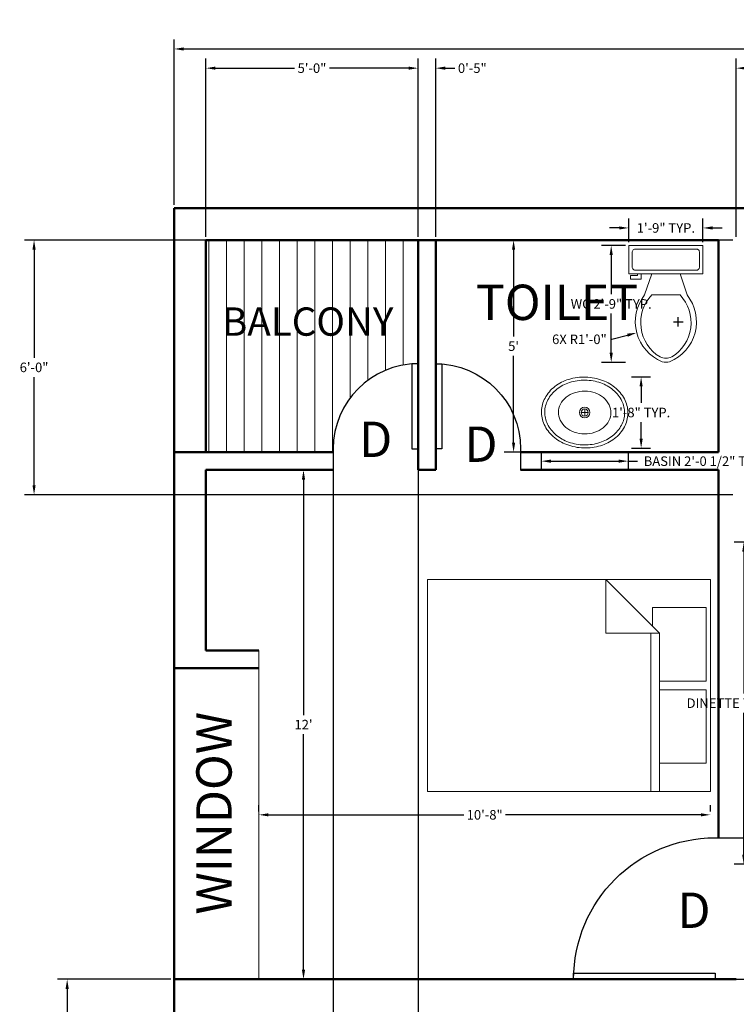
# Model space of a CAD drawing. Units: inches. Extents: x -15 to 796, y 111 to 651.
# Tile 3 of 6: x -13 to 189, y 373 to 651. Entities that reach past the tile are written whole.
import ezdxf

# ---------------------------------------------------------------- set-up
doc = ezdxf.new("R2010")
doc.units = ezdxf.units.IN
doc.header["$MEASUREMENT"] = 0
doc.layers.get('0').update_dxf_attribs({"color": 1})
for name, color, linetype, lineweight in [('A-ANNO-DIMS', 2, 'Continuous', 18), ('A-ANNO-TEXT', 7, 'Continuous', 18), ('A-AREA-IDEN', 7, 'Continuous', 25), ('A-DOOR', 3, 'Continuous', 25), ('A-FLOR-FIXT', 9, 'Continuous', 20), ('A-FLOR-PATT', 18, 'Continuous', 13), ('A-FURN', 8, 'Continuous', 18), ('A-GLAZ', 4, 'Continuous', 18), ('A-WALL', 7, 'Continuous', 50)]:
    doc.layers.add(name, color=color, linetype=linetype, lineweight=lineweight)
doc.styles.get("Standard").update_dxf_attribs({"font": 'arial.ttf'})
doc.dimstyles.get("Standard").update_dxf_attribs({"dimscale": 15, "dimtxt": 0.18, "dimasz": 0.18, "dimexe": 0.18, "dimexo": 0.0625, "dimgap": 0.09, "dimtad": 0, "dimtih": 1, "dimtoh": 1, "dimdec": 0, "dimzin": 0, "dimdsep": 46, "dimlunit": 3, "dimtxsty": 'Standard', "dimcen": 0.09, "dimadec": 0, "dimazin": 0, "dimtfac": 1, "dimtdec": 0, "dimtofl": 0, "dimtmove": 0, "dimatfit": 3, "dimfxl": 1, "dimtolj": 1, "dimtzin": 0, "dimarcsym": 0})

# ---------------------------------------------------------------- blocks, each defined once
blk = doc.blocks.new('Bed - Queen')
for p, q in [((0, -80.00003), (0, 0)), ((0, 0), (59.99999, 0)), ((59.99999, 0), (59.99999, -80.00003)), ((7.99999, -1.2), (28.79998, -1.2)), ((7.99999, -14.4), (7.99999, -1.2)), ((28.79998, -1.2), (28.79998, -14.4)), ((31.19999, -1.2), (51.99999, -1.2)), ((31.19999, -14.4), (31.19999, -1.2)), ((51.99999, -1.2), (51.99999, -16.4)), ((0, -14.4), (44.8, -14.4)), ((59.99999, -29.6), (44.8, -14.4)), ((44.8, -14.4), (44.8, -29.6)), ((51.99999, -16.4), (46.79936, -16.4)), ((44.8, -16.8), (0, -16.8)), ((44.8, -29.6), (59.99999, -29.6)), ((59.99999, -80.00003), (0, -80.00003))]:
    blk.add_line(p, q)
blk = doc.blocks.new('*U4')
for p, q in [((0, 0), (0, -6)), ((-40, 0), (-40, -6))]:
    blk.add_line(p, q)
blk.add_lwpolyline([(0, 0), (0, 40), (-1.75, 40), (-1.75, 0)], close=True)
blk.add_arc((0, 0), 40, 90, 180)
blk = doc.blocks.new('*U8')
for p, q in [((-24, 0), (-24, -6)), ((0, 0), (0, -6))]:
    blk.add_line(p, q)
blk.add_lwpolyline([(0, 0), (0, 24), (-1.75, 24), (-1.75, 0)], close=True)
blk.add_arc((0, 0), 24, 90, 180)
blk = doc.blocks.new('Sink - Oval top')
for p, q in [((-1, 0), (1, 0)), ((0, 1), (0, -1))]:
    blk.add_line(p, q)
for points in [[(-12.23, 0.39, 0.117634), (-11.46, -3.36, 0.104469), (-8.88, -6.8, 0.090016), (-5.08, -9.07, 0.08192), (-0.32, -10.02, 0.08192), (4.49, -9.38, 0.090016), (8.42, -7.36, 0.104469), (11.22, -4.09, 0.117634), (12.23, -0.39, 0.117634), (11.46, 3.36, 0.104469), (8.88, 6.8, 0.090016), (5.08, 9.07, 0.08192), (0.32, 10.02, 0.08192), (-4.49, 9.38, 0.090016), (-8.42, 7.36, 0.104469), (-11.22, 4.09, 0.117634)], [(-11.29, 0.16, 0.118622), (-10.52, -3.25, 0.104678), (-8.07, -6.36, 0.089562), (-4.54, -8.37, 0.081185), (-0.13, -9.15, 0.081185), (4.3, -8.49, 0.089562), (7.89, -6.58, 0.104678), (10.42, -3.55, 0.118622), (11.29, -0.16, 0.118622), (10.52, 3.25, 0.104678), (8.07, 6.36, 0.089562), (4.54, 8.37, 0.081185), (0.13, 9.15, 0.081185), (-4.3, 8.49, 0.089562), (-7.89, 6.58, 0.104678), (-10.42, 3.55, 0.118622)], [(-7.42, 0.08, 0.118283), (-6.91, -2.17, 0.104607), (-5.29, -4.21, 0.089718), (-2.97, -5.53, 0.081436), (-0.07, -6.04, 0.081436), (2.84, -5.59, 0.089718), (5.2, -4.33, 0.104607), (6.86, -2.32, 0.118283), (7.42, -0.08, 0.118283), (6.91, 2.17, 0.104607), (5.29, 4.21, 0.089718), (2.97, 5.53, 0.081436), (0.07, 6.04, 0.081436), (-2.84, 5.59, 0.089718), (-5.2, 4.33, 0.104607), (-6.86, 2.32, 0.118283)]]:
    blk.add_lwpolyline(points, format="xyb", close=True)
for radius in [1.5, 1]:
    blk.add_circle((0, 0), radius)
blk = doc.blocks.new('Toilet - top')
for p, q in [((9.5, -6), (9.5, -2)), ((-8, -8.5), (-8, -8)), ((-7, -8), (-7, -9.5)), ((-4, -8), (-6, -14)), ((4, -8), (6, -14)), ((-10, -8.5), (-8, -8.5)), ((-10, -9.5), (-10, -8.5)), ((-7, -9.5), (-10, -9.5)), ((4, -14), (-4, -14))]:
    blk.add_line(p, q)
blk.add_lwpolyline([(10.5, -8), (10.5, 0), (-10.5, 0), (-10.5, -8)], close=True)
for points in [[(-9.5, -2), (-9.5, -6)], [(8.5, -1), (-8.5, -1)], [(-8.5, -7), (8.5, -7)]]:
    blk.add_lwpolyline(points)
for centre, radius, start, end in [((-8.62, -1.88), 0.884, 81.8699, 188.1301), ((8.62, -1.88), 0.884, 351.8699, 98.1301), ((-8.62, -6.12), 0.884, 171.8699, 278.1301), ((8.62, -6.12), 0.884, 261.8699, 8.1301), ((3.52, -21.58), 12.17, 141.4691, 247.9714), ((4.2, -21.82), 11.33, 136.3677, 238.9468), ((-3.52, -21.58), 12.17, 292.0284, 38.5307), ((-4.2, -21.82), 11.33, 301.053, 43.6321), ((0, -27.88), 4, 245.7318, 294.2682), ((0, -29), 4, 254.8605, 285.1395)]:
    blk.add_arc(centre, radius, start, end)
blk = doc.blocks.new('*D16')
at = {"layer": 'A-ANNO-DIMS', "color": 0, "lineweight": -2, "transparency": 16777216}
for p, q in [((30.18, 599.06), (30.18, 645.85)), ((697.18, 599.06), (697.18, 645.85)), ((32.88, 643.15), (336.57, 643.15)), ((694.48, 643.15), (390.8, 643.15))]:
    blk.add_line(p, q, dxfattribs=at)
at = {"layer": 'A-ANNO-DIMS', "color": 0, "transparency": 16777216}
for points in [[(32.88, 643.6), (32.88, 642.7), (30.18, 643.15)], [(694.48, 643.6), (694.48, 642.7), (697.18, 643.15)]]:
    blk.add_solid(points, dxfattribs=at)
at = {"layer": 'Defpoints', "color": 0, "transparency": 16777216}
for p in [(697.18, 643.15), (30.18, 598.13), (697.18, 598.13)]:
    blk.add_point(p, dxfattribs=at)
at = {"layer": 'A-ANNO-DIMS', "color": 0, "transparency": 16777216, "insert": (363.68, 643.15), "char_height": 2.7, "attachment_point": 5}
blk.add_mtext('\\A1;{\\H5.55556x;55\'-7"}', dxfattribs=at)
blk = doc.blocks.new('*D19')
at = {"layer": 'A-ANNO-DIMS', "color": 0, "lineweight": -2, "transparency": 16777216}
for p, q in [((29.24, 380.13), (-2.76, 380.13)), ((-0.06, 377.43), (-0.06, 306.36)), ((-0.06, 229.83), (-0.06, 300.9)), ((29.24, 227.13), (-2.76, 227.13))]:
    blk.add_line(p, q, dxfattribs=at)
at = {"layer": 'A-ANNO-DIMS', "color": 0, "transparency": 16777216}
for points in [[(-0.51, 377.43), (0.39, 377.43), (-0.06, 380.13)], [(-0.51, 229.83), (0.39, 229.83), (-0.06, 227.13)]]:
    blk.add_solid(points, dxfattribs=at)
at = {"layer": 'Defpoints', "color": 0, "transparency": 16777216}
for p in [(30.18, 380.13), (-0.06, 227.13), (30.18, 227.13)]:
    blk.add_point(p, dxfattribs=at)
at = {"layer": 'A-ANNO-DIMS', "color": 0, "transparency": 16777216, "insert": (-0.06, 303.63), "char_height": 2.7, "attachment_point": 5}
blk.add_mtext('\\A1;12\'-9"', dxfattribs=at)
blk = doc.blocks.new('*D23')
at = {"layer": 'A-ANNO-DIMS', "color": 0, "lineweight": -2, "transparency": 16777216}
for p, q in [((141.7, 589.13), (123.49, 589.13)), ((126.19, 586.43), (126.19, 561.85)), ((126.19, 531.83), (126.19, 556.4)), ((141.7, 529.13), (123.49, 529.13))]:
    blk.add_line(p, q, dxfattribs=at)
at = {"layer": 'A-ANNO-DIMS', "color": 0, "transparency": 16777216}
for points in [[(125.74, 586.43), (126.64, 586.43), (126.19, 589.13)], [(125.74, 531.83), (126.64, 531.83), (126.19, 529.13)]]:
    blk.add_solid(points, dxfattribs=at)
at = {"layer": 'Defpoints', "color": 0, "transparency": 16777216}
for p in [(142.63, 589.13), (126.19, 529.13), (142.63, 529.13)]:
    blk.add_point(p, dxfattribs=at)
at = {"layer": 'A-ANNO-DIMS', "color": 0, "transparency": 16777216, "insert": (126.19, 559.13), "char_height": 2.7, "attachment_point": 5}
blk.add_mtext("\\A1;5'", dxfattribs=at)
blk = doc.blocks.new('*D24')
at = {"layer": 'A-ANNO-DIMS', "color": 0, "lineweight": -2, "transparency": 16777216}
for p, q in [((74.24, 524.13), (64.08, 524.13)), ((66.78, 521.43), (66.78, 454.83)), ((66.78, 382.83), (66.78, 449.42)), ((74.24, 380.13), (64.08, 380.13))]:
    blk.add_line(p, q, dxfattribs=at)
at = {"layer": 'A-ANNO-DIMS', "color": 0, "transparency": 16777216}
for points in [[(66.33, 521.43), (67.23, 521.43), (66.78, 524.13)], [(66.33, 382.83), (67.23, 382.83), (66.78, 380.13)]]:
    blk.add_solid(points, dxfattribs=at)
at = {"layer": 'Defpoints', "color": 0, "transparency": 16777216}
for p in [(75.18, 524.13), (66.78, 380.13), (75.18, 380.13)]:
    blk.add_point(p, dxfattribs=at)
at = {"layer": 'A-ANNO-DIMS', "color": 0, "transparency": 16777216, "insert": (66.78, 452.13), "char_height": 2.7, "attachment_point": 5}
blk.add_mtext("\\A1;12'", dxfattribs=at)
blk = doc.blocks.new('*D25')
at = {"layer": 'A-ANNO-DIMS', "color": 0, "lineweight": -2, "transparency": 16777216}
for p, q in [((54.18, 427.56), (54.18, 429.33)), ((181.85, 427.56), (181.85, 429.33)), ((56.88, 426.63), (112.16, 426.63)), ((179.15, 426.63), (123.88, 426.63))]:
    blk.add_line(p, q, dxfattribs=at)
at = {"layer": 'A-ANNO-DIMS', "color": 0, "transparency": 16777216}
for points in [[(56.88, 427.08), (56.88, 426.18), (54.18, 426.63)], [(179.15, 427.08), (179.15, 426.18), (181.85, 426.63)]]:
    blk.add_solid(points, dxfattribs=at)
at = {"layer": 'Defpoints', "color": 0, "transparency": 16777216}
for p in [(54.18, 426.63), (181.85, 426.63), (181.85, 426.63)]:
    blk.add_point(p, dxfattribs=at)
at = {"layer": 'A-ANNO-DIMS', "color": 0, "transparency": 16777216, "insert": (118.02, 426.63), "char_height": 2.7, "attachment_point": 5}
blk.add_mtext('\\A1;10\'-8"', dxfattribs=at)
blk = doc.blocks.new('*D45')
at = {"layer": 'A-ANNO-DIMS', "color": 0, "lineweight": -2, "transparency": 16777216}
for p, q in [((134.03, 529.37), (134.03, 523.92)), ((158.58, 529.37), (158.58, 523.92)), ((136.73, 526.62), (155.88, 526.62)), ((158.58, 526.62), (161.28, 526.62))]:
    blk.add_line(p, q, dxfattribs=at)
at = {"layer": 'A-ANNO-DIMS', "color": 0, "transparency": 16777216}
for points in [[(136.73, 527.07), (136.73, 526.17), (134.03, 526.62)], [(155.88, 527.07), (155.88, 526.17), (158.58, 526.62)]]:
    blk.add_solid(points, dxfattribs=at)
at = {"layer": 'Defpoints', "color": 0, "transparency": 16777216}
for p in [(134.03, 530.3), (158.58, 530.3), (158.58, 526.62)]:
    blk.add_point(p, dxfattribs=at)
at = {"layer": 'A-ANNO-DIMS', "color": 0, "transparency": 16777216, "insert": (180.13, 526.62), "char_height": 2.7, "attachment_point": 5}
blk.add_mtext('\\A1;BASIN 2\'-0 1/2" TYP.', dxfattribs=at)
blk = doc.blocks.new('*D46')
at = {"layer": 'A-ANNO-DIMS', "color": 0, "lineweight": -2, "transparency": 16777216}
for p, q in [((159.51, 550.44), (164.96, 550.44)), ((162.26, 547.74), (162.26, 543.1)), ((162.26, 533), (162.26, 537.64)), ((159.51, 530.3), (164.96, 530.3))]:
    blk.add_line(p, q, dxfattribs=at)
at = {"layer": 'A-ANNO-DIMS', "color": 0, "transparency": 16777216}
for points in [[(161.81, 547.74), (162.71, 547.74), (162.26, 550.44)], [(161.81, 533), (162.71, 533), (162.26, 530.3)]]:
    blk.add_solid(points, dxfattribs=at)
at = {"layer": 'Defpoints', "color": 0, "transparency": 16777216}
for p in [(158.58, 550.44), (162.26, 550.44), (158.58, 530.3)]:
    blk.add_point(p, dxfattribs=at)
at = {"layer": 'A-ANNO-DIMS', "color": 0, "transparency": 16777216, "insert": (162.26, 540.37), "char_height": 2.7, "attachment_point": 5}
blk.add_mtext('\\A1;1\'-8" TYP.', dxfattribs=at)
blk = doc.blocks.new('*D47')
at = {"layer": 'A-ANNO-DIMS', "color": 0, "lineweight": -2, "transparency": 16777216}
for p, q in [((157.82, 587.6), (151.1, 587.6)), ((153.8, 584.9), (153.8, 573.82)), ((153.8, 557.25), (153.8, 568.33)), ((157.82, 554.55), (151.1, 554.55))]:
    blk.add_line(p, q, dxfattribs=at)
at = {"layer": 'A-ANNO-DIMS', "color": 0, "transparency": 16777216}
for points in [[(153.35, 584.9), (154.25, 584.9), (153.8, 587.6)], [(153.35, 557.25), (154.25, 557.25), (153.8, 554.55)]]:
    blk.add_solid(points, dxfattribs=at)
at = {"layer": 'Defpoints', "color": 0, "transparency": 16777216}
for p in [(153.8, 587.6), (158.76, 587.6), (158.76, 554.55)]:
    blk.add_point(p, dxfattribs=at)
at = {"layer": 'A-ANNO-DIMS', "color": 0, "transparency": 16777216, "insert": (153.8, 571.07), "char_height": 2.7, "attachment_point": 5}
blk.add_mtext('\\A1;WC 2\'-9" TYP.', dxfattribs=at)
blk = doc.blocks.new('*D48')
at = {"layer": 'A-ANNO-DIMS', "color": 0, "lineweight": -2, "transparency": 16777216}
for p, q in [((158.76, 588.54), (158.76, 595.25)), ((179.76, 588.54), (179.76, 595.25)), ((156.06, 592.55), (153.36, 592.55)), ((182.46, 592.55), (185.16, 592.55))]:
    blk.add_line(p, q, dxfattribs=at)
at = {"layer": 'A-ANNO-DIMS', "color": 0, "transparency": 16777216}
for points in [[(156.06, 593), (156.06, 592.1), (158.76, 592.55)], [(182.46, 593), (182.46, 592.1), (179.76, 592.55)]]:
    blk.add_solid(points, dxfattribs=at)
at = {"layer": 'Defpoints', "color": 0, "transparency": 16777216}
for p in [(179.76, 592.55), (158.76, 587.6), (179.76, 587.6)]:
    blk.add_point(p, dxfattribs=at)
at = {"layer": 'A-ANNO-DIMS', "color": 0, "transparency": 16777216, "insert": (169.26, 592.55), "char_height": 2.7, "attachment_point": 5}
blk.add_mtext('\\A1;1\'-9" TYP.', dxfattribs=at)
blk = doc.blocks.new('*D55')
at = {"layer": 'A-ANNO-DIMS', "color": 0, "lineweight": -2, "transparency": 16777216}
for p, q in [((204, 503.69), (188.59, 503.69)), ((191.29, 500.99), (191.29, 460.89)), ((191.29, 415.39), (191.29, 455.48)), ((204, 412.69), (188.59, 412.69))]:
    blk.add_line(p, q, dxfattribs=at)
at = {"layer": 'A-ANNO-DIMS', "color": 0, "transparency": 16777216}
for points in [[(190.84, 500.99), (191.74, 500.99), (191.29, 503.69)], [(190.84, 415.39), (191.74, 415.39), (191.29, 412.69)]]:
    blk.add_solid(points, dxfattribs=at)
at = {"layer": 'Defpoints', "color": 0, "transparency": 16777216}
for p in [(204.94, 503.69), (191.29, 412.69), (204.94, 412.69)]:
    blk.add_point(p, dxfattribs=at)
at = {"layer": 'A-ANNO-DIMS', "color": 0, "transparency": 16777216, "insert": (191.29, 458.19), "char_height": 2.7, "attachment_point": 5}
blk.add_mtext('\\A1;DINETTE 7\'-7" TYP.', dxfattribs=at)
blk = doc.blocks.new('*D70')
at = {"layer": 'A-ANNO-DIMS', "color": 0, "lineweight": -2, "transparency": 16777216}
for p, q in [((39.18, 590.06), (39.18, 640.43)), ((99.18, 590.06), (99.18, 640.43)), ((41.88, 637.73), (64.24, 637.73)), ((96.48, 637.73), (74.12, 637.73))]:
    blk.add_line(p, q, dxfattribs=at)
at = {"layer": 'A-ANNO-DIMS', "color": 0, "transparency": 16777216}
for points in [[(41.88, 638.18), (41.88, 637.28), (39.18, 637.73)], [(96.48, 638.18), (96.48, 637.28), (99.18, 637.73)]]:
    blk.add_solid(points, dxfattribs=at)
at = {"layer": 'Defpoints', "color": 0, "transparency": 16777216}
for p in [(99.18, 637.73), (39.18, 589.13), (99.18, 589.13)]:
    blk.add_point(p, dxfattribs=at)
at = {"layer": 'A-ANNO-DIMS', "color": 0, "transparency": 16777216, "insert": (69.18, 637.73), "char_height": 2.7, "attachment_point": 5}
blk.add_mtext('\\A1;5\'-0"', dxfattribs=at)
blk = doc.blocks.new('*D71')
at = {"layer": 'A-ANNO-DIMS', "color": 0, "lineweight": -2, "transparency": 16777216}
for p, q in [((188.24, 589.13), (-12.12, 589.13)), ((-9.42, 586.43), (-9.42, 555.86)), ((-9.42, 519.83), (-9.42, 550.4)), ((188.24, 517.13), (-12.12, 517.13))]:
    blk.add_line(p, q, dxfattribs=at)
at = {"layer": 'A-ANNO-DIMS', "color": 0, "transparency": 16777216}
for points in [[(-9.87, 586.43), (-8.97, 586.43), (-9.42, 589.13)], [(-9.87, 519.83), (-8.97, 519.83), (-9.42, 517.13)]]:
    blk.add_solid(points, dxfattribs=at)
at = {"layer": 'Defpoints', "color": 0, "transparency": 16777216}
for p in [(189.18, 589.13), (-9.42, 517.13), (189.18, 517.13)]:
    blk.add_point(p, dxfattribs=at)
at = {"layer": 'A-ANNO-DIMS', "color": 0, "transparency": 16777216, "insert": (-9.42, 553.13), "char_height": 2.7, "attachment_point": 5}
blk.add_mtext('\\A1;6\'-0"', dxfattribs=at)
blk = doc.blocks.new('*D76')
at = {"layer": 'A-ANNO-DIMS', "color": 0, "lineweight": -2, "transparency": 16777216}
for p, q in [((189.18, 590.06), (189.18, 640.43)), ((231.37, 599.06), (231.37, 640.43)), ((191.88, 637.73), (205.34, 637.73)), ((228.67, 637.73), (215.21, 637.73))]:
    blk.add_line(p, q, dxfattribs=at)
at = {"layer": 'A-ANNO-DIMS', "color": 0, "transparency": 16777216}
for points in [[(191.88, 638.18), (191.88, 637.28), (189.18, 637.73)], [(228.67, 638.18), (228.67, 637.28), (231.37, 637.73)]]:
    blk.add_solid(points, dxfattribs=at)
at = {"layer": 'Defpoints', "color": 0, "transparency": 16777216}
for p in [(231.37, 637.73), (231.37, 598.13), (189.18, 589.13)]:
    blk.add_point(p, dxfattribs=at)
at = {"layer": 'A-ANNO-DIMS', "color": 0, "transparency": 16777216, "insert": (210.27, 637.73), "char_height": 2.7, "attachment_point": 5}
blk.add_mtext('\\A1;3\'-6"', dxfattribs=at)
blk = doc.blocks.new('*D78')
at = {"layer": 'A-ANNO-DIMS', "color": 0, "lineweight": -2, "transparency": 16777216}
for p, q in [((185.12, 420.13), (739.48, 420.13)), ((736.78, 417.43), (736.78, 402.86)), ((736.78, 382.83), (736.78, 397.4)), ((185.87, 380.13), (739.48, 380.13))]:
    blk.add_line(p, q, dxfattribs=at)
at = {"layer": 'A-ANNO-DIMS', "color": 0, "transparency": 16777216}
for points in [[(736.33, 417.43), (737.23, 417.43), (736.78, 420.13)], [(736.33, 382.83), (737.23, 382.83), (736.78, 380.13)]]:
    blk.add_solid(points, dxfattribs=at)
at = {"layer": 'Defpoints', "color": 0, "transparency": 16777216}
for p in [(184.18, 420.13), (736.78, 420.13), (184.93, 380.13)]:
    blk.add_point(p, dxfattribs=at)
at = {"layer": 'A-ANNO-DIMS', "color": 0, "transparency": 16777216, "insert": (736.78, 400.13), "char_height": 2.7, "attachment_point": 5}
blk.add_mtext('\\A1;3\'-4"', dxfattribs=at)
blk = doc.blocks.new('*D80')
at = {"layer": 'A-ANNO-DIMS', "color": 0, "lineweight": -2, "transparency": 16777216}
for p, q in [((75.18, 528.19), (75.18, 125.83)), ((99.18, 527.44), (99.18, 125.83)), ((77.88, 128.53), (82.22, 128.53)), ((96.48, 128.53), (92.14, 128.53))]:
    blk.add_line(p, q, dxfattribs=at)
at = {"layer": 'A-ANNO-DIMS', "color": 0, "transparency": 16777216}
for points in [[(77.88, 128.98), (77.88, 128.08), (75.18, 128.53)], [(96.48, 128.98), (96.48, 128.08), (99.18, 128.53)]]:
    blk.add_solid(points, dxfattribs=at)
at = {"layer": 'Defpoints', "color": 0, "transparency": 16777216}
for p in [(75.18, 529.13), (99.18, 528.38), (75.18, 128.53)]:
    blk.add_point(p, dxfattribs=at)
at = {"layer": 'A-ANNO-DIMS', "color": 0, "transparency": 16777216, "insert": (87.18, 128.53), "char_height": 2.7, "attachment_point": 5}
blk.add_mtext('\\A1;2\'-0"', dxfattribs=at)
blk = doc.blocks.new('*D82')
at = {"layer": 'A-ANNO-DIMS', "color": 0, "lineweight": -2, "transparency": 16777216}
for p, q in [((99.18, 590.06), (99.18, 640.43)), ((104.18, 590.06), (104.18, 640.43)), ((96.48, 637.73), (93.78, 637.73)), ((106.88, 637.73), (109.58, 637.73))]:
    blk.add_line(p, q, dxfattribs=at)
at = {"layer": 'A-ANNO-DIMS', "color": 0, "transparency": 16777216}
for points in [[(96.48, 638.18), (96.48, 637.28), (99.18, 637.73)], [(106.88, 638.18), (106.88, 637.28), (104.18, 637.73)]]:
    blk.add_solid(points, dxfattribs=at)
at = {"layer": 'Defpoints', "color": 0, "transparency": 16777216}
for p in [(104.18, 637.73), (99.18, 589.13), (104.18, 589.13)]:
    blk.add_point(p, dxfattribs=at)
at = {"layer": 'A-ANNO-DIMS', "color": 0, "transparency": 16777216, "insert": (114.52, 637.73), "char_height": 2.7, "attachment_point": 5}
blk.add_mtext('\\A1;0\'-5"', dxfattribs=at)
blk = doc.blocks.new('*D89')
at = {"layer": 'A-ANNO-DIMS', "color": 0, "lineweight": -2, "transparency": 16777216}
for p, q in [((171.43, 566.02), (174.13, 566.02)), ((172.78, 564.67), (172.78, 567.37)), ((153.95, 561.07), (158.4, 562.24))]:
    blk.add_line(p, q, dxfattribs=at)
at = {"layer": 'A-ANNO-DIMS', "color": 0, "transparency": 16777216}
blk.add_solid([(158.28, 562.67), (158.51, 561.8), (161.01, 562.92)], dxfattribs=at)
at = {"layer": 'Defpoints', "color": 0, "transparency": 16777216}
for p in [(172.78, 566.02), (161.01, 562.92)]:
    blk.add_point(p, dxfattribs=at)
at = {"layer": 'A-ANNO-DIMS', "color": 0, "transparency": 16777216, "insert": (144.81, 561.07), "char_height": 2.7, "attachment_point": 5}
blk.add_mtext('\\A1;6X R1\'-0"', dxfattribs=at)

msp = doc.modelspace()

# ---------------------------------------------------------------- hatches: boundary and pattern name
at = {"layer": 'A-FLOR-PATT'}
h = msp.add_hatch(dxfattribs=at)
h.set_pattern_fill('_USER', color=256, scale=5, angle=90, pattern_type=0)
h.set_pattern_definition([(90, (0, 0), (-5, 3e-16), [])])
h.paths.add_polyline_path([(99.18, 589.13), (39.18, 589.13), (39.18, 529.13), (75.18, 529.13), (75.18, 530.13, -0.392996), (97.43, 554.06), (97.43, 554.13), (99.18, 554.13)])
h.paths.add_polyline_path([(688.18, 589.13), (628.18, 589.13), (628.18, 554.13), (629.93, 554.13), (629.93, 554.06, -0.392996), (652.18, 530.13), (652.18, 529.13), (688.18, 529.13)])
h.paths.add_polyline_path([(40.9, 557.57), (98.32, 557.57), (98.32, 574.06), (40.9, 574.06)], flags=24)
h.paths.add_polyline_path([(628.32, 557.57), (685.73, 557.57), (685.73, 574.06), (628.32, 574.06)], flags=24)

# ---------------------------------------------------------------- linework, layer by layer
at = {"layer": 'A-GLAZ'}
msp.add_line((54.18, 473.13), (54.18, 380.13), dxfattribs=at)
at = {"layer": 'A-WALL'}
for p, q in [((30.18, 598.13), (30.18, 468.13)), ((322.48, 598.13), (30.18, 598.13)), ((39.18, 589.13), (39.18, 529.13)), ((184.18, 589.13), (39.18, 589.13)), ((99.18, 589.13), (99.18, 524.13)), ((104.18, 589.13), (104.18, 524.13)), ((184.18, 529.13), (184.18, 589.13)), ((39.18, 529.13), (30.18, 529.13)), ((75.18, 529.13), (39.18, 529.13)), ((184.18, 529.13), (128.18, 529.13)), ((39.18, 524.13), (39.18, 473.13)), ((75.18, 524.13), (39.18, 524.13)), ((104.18, 524.13), (99.18, 524.13)), ((184.18, 524.13), (128.18, 524.13)), ((184.18, 420.13), (184.18, 524.13)), ((54.18, 473.13), (39.18, 473.13)), ((30.18, 468.13), (30.18, 380.13)), ((54.18, 468.13), (30.18, 468.13)), ((30.18, 380.13), (30.18, 227.13)), ((189.18, 380.13), (30.18, 380.13))]:
    msp.add_line(p, q, dxfattribs=at)

# ---------------------------------------------------------------- block references
at = {"layer": 'A-DOOR'}
msp.add_blockref('*U8', (99.18, 530.13), dxfattribs=at)
at = {"layer": 'A-DOOR', "xscale": -1}
msp.add_blockref('*U8', (104.18, 530.13), dxfattribs=at)
at = {"layer": 'A-DOOR', "xscale": -1, "rotation": 90}
msp.add_blockref('*U4', (183.18, 380.13), dxfattribs=at)
at = {"layer": 'A-FLOR-FIXT'}
for name, p in [('Toilet - top', (169.26, 587.6)), ('Sink - Oval top', (146.3, 540.37))]:
    msp.add_blockref(name, p, dxfattribs=at)
at = {"layer": 'A-FURN', "xscale": -1, "rotation": 270}
msp.add_blockref('Bed - Queen', (181.85, 433.2), dxfattribs=at)

# ---------------------------------------------------------------- texts
at = {"layer": 'A-ANNO-TEXT'}
msp.add_text('WINDOW', height=10, rotation=90, dxfattribs=at).set_placement((46.46, 398.41))
at = {"layer": 'A-ANNO-TEXT', "char_height": 10, "attachment_point": 1}
for insert in [(82.5, 537.79), (112.27, 536.41), (172.51, 404.64)]:
    msp.add_mtext_dynamic_manual_height_columns('D', width=13.2435, gutter_width=1, heights=[0], dxfattribs=dict(at, insert=insert))
at = {"layer": 'A-AREA-IDEN', "attachment_point": 1}
for s, width, insert, char_height in [('TOILET', 20.6028, (115.54, 576.52), 10), ('BALCONY', 13.9372, (43.72, 570.08), 8)]:
    msp.add_mtext_dynamic_manual_height_columns(s, width=width, gutter_width=50, heights=[0], dxfattribs=dict(at, insert=insert, char_height=char_height))

# ---------------------------------------------------------------- dimensions: what is measured, and where the dimension line sits
at = {"layer": 'A-ANNO-DIMS'}
dim = msp.add_linear_dim(base=(697.18, 643.15), p1=(30.18, 598.13), p2=(697.18, 598.13), text='{\\H5.55556x;<>}', dimstyle='Standard', override={"dimclrd": 0, "dimclre": 0, "dimclrt": 0}, dxfattribs=at)
dim.commit()
dim.dimension.update_dxf_attribs({"geometry": '*D16', "text_midpoint": (363.68, 643.15), "dimtype": 160})
for base, p1, p2, override, picture, middle in [((99.18, 637.73), (39.18, 589.13), (99.18, 589.13), {"dimdec": 1, "dimlfac": 1, "dimrnd": 0, "dimzin": 1, "dimdsep": 46, "dimlunit": 4, "dimfrac": 2}, '*D70', (69.18, 637.73)), ((104.18, 637.73), (99.18, 589.13), (104.18, 589.13), {"dimdec": 1, "dimlfac": 1, "dimrnd": 0, "dimzin": 1, "dimdsep": 46, "dimlunit": 4, "dimfrac": 2}, '*D82', (114.52, 637.73)), ((231.37, 637.73), (189.18, 589.13), (231.37, 598.13), {"dimdec": 1, "dimlfac": 1, "dimrnd": 0, "dimzin": 1, "dimdsep": 46, "dimlunit": 4, "dimfrac": 2}, '*D76', (210.27, 637.73)), ((75.18, 128.53), (99.18, 528.38), (75.18, 529.13), {"dimdec": 1, "dimlfac": 1, "dimrnd": 0, "dimzin": 1, "dimdsep": 46, "dimlunit": 4, "dimfrac": 2}, '*D80', (87.18, 128.53)), ((181.85, 426.63), (54.18, 426.63), (181.85, 426.63), {"dimclrd": 0, "dimclre": 0, "dimclrt": 0}, '*D25', (118.02, 426.63))]:
    dim = msp.add_linear_dim(base=base, p1=p1, p2=p2, dimstyle='Standard', override=override, dxfattribs=at)
    dim.commit()
    dim.dimension.update_dxf_attribs({"geometry": picture, "text_midpoint": middle})
for base, p1, p2, text, picture, middle in [((179.76, 592.55), (158.76, 587.6), (179.76, 587.6), '<> TYP.', '*D48', (169.26, 592.55)), ((158.5769, 526.6215), (134.026, 530.3042), (158.5769, 530.3042), 'BASIN <> TYP.', '*D45', (180.1253, 526.6215))]:
    dim = msp.add_linear_dim(base=base, p1=p1, p2=p2, text=text, dimstyle='Standard', override={"dimdec": 1, "dimlfac": 1, "dimrnd": 0, "dimzin": 1, "dimdsep": 46, "dimlunit": 4, "dimfrac": 2}, dxfattribs=at)
    dim.commit()
    dim.dimension.update_dxf_attribs({"geometry": picture, "text_midpoint": middle})
for base, p1, p2, override, picture, middle in [((-9.42, 517.13), (189.18, 589.13), (189.18, 517.13), {"dimdec": 1, "dimlfac": 1, "dimrnd": 0, "dimzin": 1, "dimdsep": 46, "dimlunit": 4, "dimfrac": 2}, '*D71', (-9.42, 553.13)), ((126.19, 529.13), (142.63, 589.13), (142.63, 529.13), {"dimclrd": 0, "dimclre": 0, "dimclrt": 0}, '*D23', (126.19, 559.13)), ((66.78, 380.13), (75.18, 524.13), (75.18, 380.13), {"dimclrd": 0, "dimclre": 0, "dimclrt": 0}, '*D24', (66.78, 452.13)), ((736.78, 420.13), (184.93, 380.13), (184.18, 420.13), {"dimdec": 1, "dimlfac": 1, "dimrnd": 0, "dimzin": 1, "dimdsep": 46, "dimlunit": 4, "dimfrac": 2}, '*D78', (736.78, 400.13)), ((-0.06, 227.13), (30.18, 380.13), (30.18, 227.13), {"dimclrd": 0, "dimclre": 0, "dimclrt": 0}, '*D19', (-0.06, 303.63))]:
    dim = msp.add_linear_dim(base=base, p1=p1, p2=p2, angle=90, dimstyle='Standard', override=override, dxfattribs=at)
    dim.commit()
    dim.dimension.update_dxf_attribs({"geometry": picture, "text_midpoint": middle})
for base, p1, p2, angle, text, picture, middle in [((153.8028, 587.5979), (158.7598, 554.5517), (158.7598, 587.5979), 90, 'WC <> TYP.', '*D47', (153.8028, 571.0748)), ((162.26, 550.44), (158.58, 530.3), (158.58, 550.44), 90, '<> TYP.', '*D46', (162.26, 540.37)), ((191.29, 412.69), (204.94, 503.69), (204.94, 412.69), 270, 'DINETTE <> TYP.', '*D55', (191.29, 458.19))]:
    dim = msp.add_linear_dim(base=base, p1=p1, p2=p2, angle=angle, text=text, dimstyle='Standard', override={"dimdec": 1, "dimlfac": 1, "dimrnd": 0, "dimzin": 1, "dimdsep": 46, "dimlunit": 4, "dimfrac": 2}, dxfattribs=at)
    dim.commit()
    dim.dimension.update_dxf_attribs({"geometry": picture, "text_midpoint": middle})
dim = msp.add_radius_dim(center=(172.78, 566.02), mpoint=(161.01, 562.92), text='6X <>', dimstyle='Standard', override={"dimdec": 1, "dimlfac": 1, "dimrnd": 0, "dimzin": 1, "dimdsep": 46, "dimlunit": 4, "dimfrac": 2}, dxfattribs=at)
dim.commit()
dim.dimension.update_dxf_attribs({"geometry": '*D89', "text_midpoint": (153.95, 561.07), "dimtype": 164})

doc.saveas('drawing.dxf')
